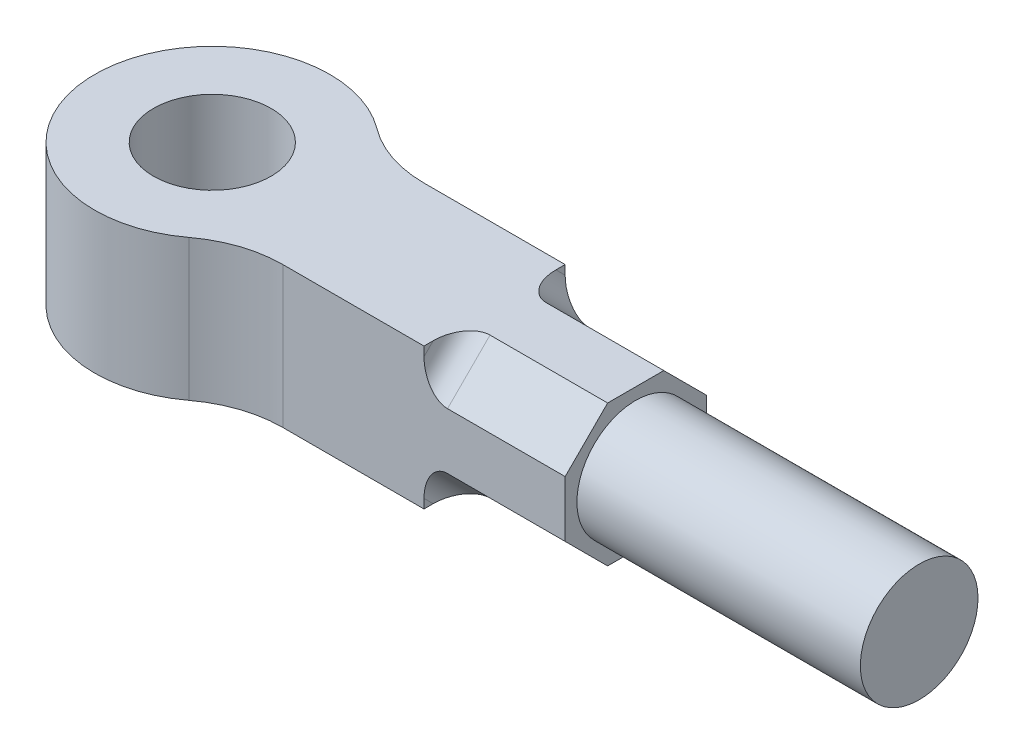
ISO-10303-21;
HEADER;
FILE_DESCRIPTION(('STEP AP214'),'2;1');
FILE_NAME('part.step','',(''),(''),'','','');
FILE_SCHEMA(('AUTOMOTIVE_DESIGN { 1 0 10303 214 1 1 1 1 }'));
ENDSEC;
DATA;
#1=APPLICATION_CONTEXT('core data for automotive mechanical design processes');
#2=APPLICATION_PROTOCOL_DEFINITION('international standard','automotive_design',2000,#1);
#3=PRODUCT_CONTEXT('',#1,'mechanical');
#4=PRODUCT('Part','Part','',(#3));
#5=PRODUCT_RELATED_PRODUCT_CATEGORY('part','',(#4));
#6=PRODUCT_DEFINITION_FORMATION('','',#4);
#7=PRODUCT_DEFINITION_CONTEXT('part definition',#1,'design');
#8=PRODUCT_DEFINITION('design','',#6,#7);
#9=PRODUCT_DEFINITION_SHAPE('','',#8);
#10=(LENGTH_UNIT() NAMED_UNIT(*) SI_UNIT(.MILLI.,.METRE.));
#11=(NAMED_UNIT(*) PLANE_ANGLE_UNIT() SI_UNIT($,.RADIAN.));
#12=(NAMED_UNIT(*) SI_UNIT($,.STERADIAN.) SOLID_ANGLE_UNIT());
#13=UNCERTAINTY_MEASURE_WITH_UNIT(LENGTH_MEASURE(1.E-05),#10,'distance_accuracy_value','');
#14=(GEOMETRIC_REPRESENTATION_CONTEXT(3) GLOBAL_UNCERTAINTY_ASSIGNED_CONTEXT((#13)) GLOBAL_UNIT_ASSIGNED_CONTEXT((#10,
#11,#12)) REPRESENTATION_CONTEXT('',''));
#15=CARTESIAN_POINT('',(0.,0.,0.));
#16=DIRECTION('',(0.,0.,1.));
#17=DIRECTION('',(1.,0.,0.));
#18=AXIS2_PLACEMENT_3D('',#15,#16,#17);
#19=CARTESIAN_POINT('',(60.,60.,-80.));
#20=DIRECTION('',(0.,1.,0.));
#21=DIRECTION('',(0.,0.,1.));
#22=AXIS2_PLACEMENT_3D('',#19,#20,#21);
#23=PLANE('',#22);
#24=CARTESIAN_POINT('',(0.,60.,0.));
#25=DIRECTION('',(0.,1.,0.));
#26=DIRECTION('',(0.,0.,1.));
#27=AXIS2_PLACEMENT_3D('',#24,#25,#26);
#28=CIRCLE('',#27,25.);
#29=CARTESIAN_POINT('',(0.,60.,25.));
#30=VERTEX_POINT('',#29);
#31=EDGE_CURVE('E289',#30,#30,#28,.T.);
#32=ORIENTED_EDGE('',*,*,#31,.F.);
#33=EDGE_LOOP('',(#32));
#34=FACE_BOUND('',#33,.T.);
#35=DIRECTION('',(0.,0.,-1.));
#36=VECTOR('',#35,1.);
#37=CARTESIAN_POINT('',(180.,60.,-30.));
#38=LINE('',#37,#36);
#39=CARTESIAN_POINT('',(180.,60.,11.9399999999999));
#40=VERTEX_POINT('',#39);
#41=CARTESIAN_POINT('',(180.,60.,-11.94));
#42=VERTEX_POINT('',#41);
#43=EDGE_CURVE('E303',#40,#42,#38,.T.);
#44=ORIENTED_EDGE('',*,*,#43,.T.);
#45=DIRECTION('',(1.,0.,0.));
#46=VECTOR('',#45,1.);
#47=CARTESIAN_POINT('',(120.,60.,-11.94));
#48=LINE('',#47,#46);
#49=CARTESIAN_POINT('',(130.,60.,-11.94));
#50=VERTEX_POINT('',#49);
#51=EDGE_CURVE('E290',#50,#42,#48,.T.);
#52=ORIENTED_EDGE('',*,*,#51,.F.);
#53=CARTESIAN_POINT('',(130.,60.,-26.0821356237309));
#54=DIRECTION('',(0.,1.,0.));
#55=DIRECTION('',(0.,0.,-1.));
#56=AXIS2_PLACEMENT_3D('',#53,#54,#55);
#57=ELLIPSE('',#56,14.1421356237309,10.);
#58=CARTESIAN_POINT('',(120.,60.,-26.0821356237309));
#59=VERTEX_POINT('',#58);
#60=EDGE_CURVE('E47',#50,#59,#57,.F.);
#61=ORIENTED_EDGE('',*,*,#60,.T.);
#62=DIRECTION('',(0.,0.,1.));
#63=VECTOR('',#62,1.);
#64=CARTESIAN_POINT('',(120.,60.,0.));
#65=LINE('',#64,#63);
#66=CARTESIAN_POINT('',(120.,60.,-30.));
#67=VERTEX_POINT('',#66);
#68=EDGE_CURVE('E333',#67,#59,#65,.T.);
#69=ORIENTED_EDGE('',*,*,#68,.F.);
#70=DIRECTION('',(-1.,0.,0.));
#71=VECTOR('',#70,1.);
#72=CARTESIAN_POINT('',(60.,60.,-30.));
#73=LINE('',#72,#71);
#74=CARTESIAN_POINT('',(60.,60.,-30.));
#75=VERTEX_POINT('',#74);
#76=EDGE_CURVE('E209',#67,#75,#73,.T.);
#77=ORIENTED_EDGE('',*,*,#76,.T.);
#78=CARTESIAN_POINT('',(60.,60.,-80.));
#79=DIRECTION('',(0.,-1.,0.));
#80=DIRECTION('',(0.,0.,1.));
#81=AXIS2_PLACEMENT_3D('',#78,#79,#80);
#82=CIRCLE('',#81,50.);
#83=CARTESIAN_POINT('',(30.,60.,-40.));
#84=VERTEX_POINT('',#83);
#85=EDGE_CURVE('E200',#75,#84,#82,.T.);
#86=ORIENTED_EDGE('',*,*,#85,.T.);
#87=CARTESIAN_POINT('',(0.,60.,0.));
#88=DIRECTION('',(0.,1.,0.));
#89=DIRECTION('',(0.,0.,1.));
#90=AXIS2_PLACEMENT_3D('',#87,#88,#89);
#91=CIRCLE('',#90,50.);
#92=CARTESIAN_POINT('',(30.,60.,40.));
#93=VERTEX_POINT('',#92);
#94=EDGE_CURVE('E296',#84,#93,#91,.T.);
#95=ORIENTED_EDGE('',*,*,#94,.T.);
#96=CARTESIAN_POINT('',(60.,60.,80.));
#97=DIRECTION('',(0.,-1.,0.));
#98=DIRECTION('',(0.,0.,-1.));
#99=AXIS2_PLACEMENT_3D('',#96,#97,#98);
#100=CIRCLE('',#99,50.);
#101=CARTESIAN_POINT('',(60.,60.,30.));
#102=VERTEX_POINT('',#101);
#103=EDGE_CURVE('E297',#93,#102,#100,.T.);
#104=ORIENTED_EDGE('',*,*,#103,.T.);
#105=DIRECTION('',(1.,0.,0.));
#106=VECTOR('',#105,1.);
#107=CARTESIAN_POINT('',(60.,60.,30.));
#108=LINE('',#107,#106);
#109=CARTESIAN_POINT('',(120.,60.,30.));
#110=VERTEX_POINT('',#109);
#111=EDGE_CURVE('E305',#102,#110,#108,.T.);
#112=ORIENTED_EDGE('',*,*,#111,.T.);
#113=DIRECTION('',(0.,0.,1.));
#114=VECTOR('',#113,1.);
#115=CARTESIAN_POINT('',(120.,60.,0.));
#116=LINE('',#115,#114);
#117=CARTESIAN_POINT('',(120.,60.,26.0821356237309));
#118=VERTEX_POINT('',#117);
#119=EDGE_CURVE('E259',#118,#110,#116,.T.);
#120=ORIENTED_EDGE('',*,*,#119,.F.);
#121=CARTESIAN_POINT('',(130.,60.,26.0821356237309));
#122=DIRECTION('',(0.,1.,0.));
#123=DIRECTION('',(0.,0.,-1.));
#124=AXIS2_PLACEMENT_3D('',#121,#122,#123);
#125=ELLIPSE('',#124,14.142135623731,10.);
#126=CARTESIAN_POINT('',(130.,60.,11.94));
#127=VERTEX_POINT('',#126);
#128=EDGE_CURVE('E253',#118,#127,#125,.F.);
#129=ORIENTED_EDGE('',*,*,#128,.T.);
#130=DIRECTION('',(1.,0.,0.));
#131=VECTOR('',#130,1.);
#132=CARTESIAN_POINT('',(120.,60.,11.94));
#133=LINE('',#132,#131);
#134=EDGE_CURVE('E258',#127,#40,#133,.T.);
#135=ORIENTED_EDGE('',*,*,#134,.T.);
#136=EDGE_LOOP('',(#44,#52,#61,#69,#77,#86,#95,#104,#112,#120,#129,#135));
#137=FACE_BOUND('',#136,.T.);
#138=ADVANCED_FACE('F41',(#34,#137),#23,.T.);
#139=CARTESIAN_POINT('',(60.,0.,-80.));
#140=DIRECTION('',(0.,1.,0.));
#141=DIRECTION('',(0.,0.,1.));
#142=AXIS2_PLACEMENT_3D('',#139,#140,#141);
#143=PLANE('',#142);
#144=CARTESIAN_POINT('',(0.,0.,0.));
#145=DIRECTION('',(0.,1.,0.));
#146=DIRECTION('',(0.,0.,1.));
#147=AXIS2_PLACEMENT_3D('',#144,#145,#146);
#148=CIRCLE('',#147,25.);
#149=CARTESIAN_POINT('',(0.,0.,25.));
#150=VERTEX_POINT('',#149);
#151=EDGE_CURVE('E287',#150,#150,#148,.T.);
#152=ORIENTED_EDGE('',*,*,#151,.T.);
#153=EDGE_LOOP('',(#152));
#154=FACE_BOUND('',#153,.T.);
#155=DIRECTION('',(1.,0.,0.));
#156=VECTOR('',#155,1.);
#157=CARTESIAN_POINT('',(120.,0.,11.94));
#158=LINE('',#157,#156);
#159=CARTESIAN_POINT('',(130.,0.,11.94));
#160=VERTEX_POINT('',#159);
#161=CARTESIAN_POINT('',(180.,0.,11.94));
#162=VERTEX_POINT('',#161);
#163=EDGE_CURVE('E324',#160,#162,#158,.T.);
#164=ORIENTED_EDGE('',*,*,#163,.F.);
#165=CARTESIAN_POINT('',(130.,0.,26.082135623731));
#166=DIRECTION('',(0.,1.,0.));
#167=DIRECTION('',(0.,0.,1.));
#168=AXIS2_PLACEMENT_3D('',#165,#166,#167);
#169=ELLIPSE('',#168,14.1421356237309,10.);
#170=CARTESIAN_POINT('',(120.,0.,26.082135623731));
#171=VERTEX_POINT('',#170);
#172=EDGE_CURVE('E242',#160,#171,#169,.T.);
#173=ORIENTED_EDGE('',*,*,#172,.T.);
#174=DIRECTION('',(0.,0.,-1.));
#175=VECTOR('',#174,1.);
#176=CARTESIAN_POINT('',(120.,0.,0.));
#177=LINE('',#176,#175);
#178=CARTESIAN_POINT('',(120.,0.,30.));
#179=VERTEX_POINT('',#178);
#180=EDGE_CURVE('E317',#179,#171,#177,.T.);
#181=ORIENTED_EDGE('',*,*,#180,.F.);
#182=DIRECTION('',(1.,0.,0.));
#183=VECTOR('',#182,1.);
#184=CARTESIAN_POINT('',(60.,0.,30.));
#185=LINE('',#184,#183);
#186=CARTESIAN_POINT('',(60.,0.,30.));
#187=VERTEX_POINT('',#186);
#188=EDGE_CURVE('E197',#187,#179,#185,.T.);
#189=ORIENTED_EDGE('',*,*,#188,.F.);
#190=CARTESIAN_POINT('',(60.,0.,80.));
#191=DIRECTION('',(0.,-1.,0.));
#192=DIRECTION('',(0.,0.,-1.));
#193=AXIS2_PLACEMENT_3D('',#190,#191,#192);
#194=CIRCLE('',#193,50.);
#195=CARTESIAN_POINT('',(30.,0.,40.));
#196=VERTEX_POINT('',#195);
#197=EDGE_CURVE('E205',#196,#187,#194,.T.);
#198=ORIENTED_EDGE('',*,*,#197,.F.);
#199=CARTESIAN_POINT('',(0.,0.,0.));
#200=DIRECTION('',(0.,1.,0.));
#201=DIRECTION('',(0.,0.,1.));
#202=AXIS2_PLACEMENT_3D('',#199,#200,#201);
#203=CIRCLE('',#202,50.);
#204=CARTESIAN_POINT('',(30.,0.,-40.));
#205=VERTEX_POINT('',#204);
#206=EDGE_CURVE('E310',#205,#196,#203,.T.);
#207=ORIENTED_EDGE('',*,*,#206,.F.);
#208=CARTESIAN_POINT('',(60.,0.,-80.));
#209=DIRECTION('',(0.,-1.,0.));
#210=DIRECTION('',(0.,0.,1.));
#211=AXIS2_PLACEMENT_3D('',#208,#209,#210);
#212=CIRCLE('',#211,50.);
#213=CARTESIAN_POINT('',(60.,0.,-30.));
#214=VERTEX_POINT('',#213);
#215=EDGE_CURVE('E291',#214,#205,#212,.T.);
#216=ORIENTED_EDGE('',*,*,#215,.F.);
#217=DIRECTION('',(-1.,0.,0.));
#218=VECTOR('',#217,1.);
#219=CARTESIAN_POINT('',(60.,0.,-30.));
#220=LINE('',#219,#218);
#221=CARTESIAN_POINT('',(120.,0.,-30.));
#222=VERTEX_POINT('',#221);
#223=EDGE_CURVE('E198',#222,#214,#220,.T.);
#224=ORIENTED_EDGE('',*,*,#223,.F.);
#225=DIRECTION('',(0.,0.,-1.));
#226=VECTOR('',#225,1.);
#227=CARTESIAN_POINT('',(120.,0.,0.));
#228=LINE('',#227,#226);
#229=CARTESIAN_POINT('',(120.,0.,-26.0821356237309));
#230=VERTEX_POINT('',#229);
#231=EDGE_CURVE('E190',#230,#222,#228,.T.);
#232=ORIENTED_EDGE('',*,*,#231,.F.);
#233=CARTESIAN_POINT('',(130.,0.,-26.0821356237309));
#234=DIRECTION('',(0.,1.,0.));
#235=DIRECTION('',(0.,0.,1.));
#236=AXIS2_PLACEMENT_3D('',#233,#234,#235);
#237=ELLIPSE('',#236,14.142135623731,10.);
#238=CARTESIAN_POINT('',(130.,0.,-11.9399999999999));
#239=VERTEX_POINT('',#238);
#240=EDGE_CURVE('E171',#230,#239,#237,.T.);
#241=ORIENTED_EDGE('',*,*,#240,.T.);
#242=DIRECTION('',(1.,0.,0.));
#243=VECTOR('',#242,1.);
#244=CARTESIAN_POINT('',(120.,0.,-11.9399999999999));
#245=LINE('',#244,#243);
#246=CARTESIAN_POINT('',(180.,0.,-11.9399999999999));
#247=VERTEX_POINT('',#246);
#248=EDGE_CURVE('E164',#239,#247,#245,.T.);
#249=ORIENTED_EDGE('',*,*,#248,.T.);
#250=DIRECTION('',(0.,0.,-1.));
#251=VECTOR('',#250,1.);
#252=CARTESIAN_POINT('',(180.,0.,-30.));
#253=LINE('',#252,#251);
#254=EDGE_CURVE('E168',#162,#247,#253,.T.);
#255=ORIENTED_EDGE('',*,*,#254,.F.);
#256=EDGE_LOOP('',(#164,#173,#181,#189,#198,#207,#216,#224,#232,#241,#249,#255));
#257=FACE_BOUND('',#256,.T.);
#258=ADVANCED_FACE('F169',(#154,#257),#143,.F.);
#259=CARTESIAN_POINT('',(60.,60.,30.));
#260=DIRECTION('',(0.,0.,-1.));
#261=DIRECTION('',(-1.,0.,0.));
#262=AXIS2_PLACEMENT_3D('',#259,#260,#261);
#263=PLANE('',#262);
#264=DIRECTION('',(0.,-1.,0.));
#265=VECTOR('',#264,1.);
#266=CARTESIAN_POINT('',(120.,0.,30.));
#267=LINE('',#266,#265);
#268=CARTESIAN_POINT('',(120.,3.91786437626909,30.));
#269=VERTEX_POINT('',#268);
#270=EDGE_CURVE('E323',#269,#179,#267,.T.);
#271=ORIENTED_EDGE('',*,*,#270,.F.);
#272=CARTESIAN_POINT('',(130.,3.91786437626906,30.));
#273=DIRECTION('',(0.,0.,-1.));
#274=DIRECTION('',(0.,1.,0.));
#275=AXIS2_PLACEMENT_3D('',#272,#273,#274);
#276=ELLIPSE('',#275,14.142135623731,10.);
#277=CARTESIAN_POINT('',(130.,18.0600000000001,30.));
#278=VERTEX_POINT('',#277);
#279=EDGE_CURVE('E250',#269,#278,#276,.T.);
#280=ORIENTED_EDGE('',*,*,#279,.T.);
#281=DIRECTION('',(1.,0.,0.));
#282=VECTOR('',#281,1.);
#283=CARTESIAN_POINT('',(120.,18.0600000000001,30.));
#284=LINE('',#283,#282);
#285=CARTESIAN_POINT('',(180.,18.0600000000001,30.));
#286=VERTEX_POINT('',#285);
#287=EDGE_CURVE('E325',#278,#286,#284,.T.);
#288=ORIENTED_EDGE('',*,*,#287,.T.);
#289=DIRECTION('',(0.,-1.,0.));
#290=VECTOR('',#289,1.);
#291=CARTESIAN_POINT('',(180.,60.,30.));
#292=LINE('',#291,#290);
#293=CARTESIAN_POINT('',(180.,41.94,30.));
#294=VERTEX_POINT('',#293);
#295=EDGE_CURVE('E215',#294,#286,#292,.T.);
#296=ORIENTED_EDGE('',*,*,#295,.F.);
#297=DIRECTION('',(1.,0.,0.));
#298=VECTOR('',#297,1.);
#299=CARTESIAN_POINT('',(120.,41.94,30.));
#300=LINE('',#299,#298);
#301=CARTESIAN_POINT('',(130.,41.94,30.));
#302=VERTEX_POINT('',#301);
#303=EDGE_CURVE('E267',#302,#294,#300,.T.);
#304=ORIENTED_EDGE('',*,*,#303,.F.);
#305=CARTESIAN_POINT('',(130.,56.0821356237309,30.));
#306=DIRECTION('',(0.,0.,-1.));
#307=DIRECTION('',(0.,1.,0.));
#308=AXIS2_PLACEMENT_3D('',#305,#306,#307);
#309=ELLIPSE('',#308,14.1421356237309,10.);
#310=CARTESIAN_POINT('',(120.,56.0821356237309,30.));
#311=VERTEX_POINT('',#310);
#312=EDGE_CURVE('E248',#302,#311,#309,.T.);
#313=ORIENTED_EDGE('',*,*,#312,.T.);
#314=DIRECTION('',(0.,-1.,0.));
#315=VECTOR('',#314,1.);
#316=CARTESIAN_POINT('',(120.,0.,30.));
#317=LINE('',#316,#315);
#318=EDGE_CURVE('E269',#110,#311,#317,.T.);
#319=ORIENTED_EDGE('',*,*,#318,.F.);
#320=ORIENTED_EDGE('',*,*,#111,.F.);
#321=DIRECTION('',(0.,-1.,0.));
#322=VECTOR('',#321,1.);
#323=CARTESIAN_POINT('',(60.,60.,30.));
#324=LINE('',#323,#322);
#325=EDGE_CURVE('E212',#102,#187,#324,.T.);
#326=ORIENTED_EDGE('',*,*,#325,.T.);
#327=ORIENTED_EDGE('',*,*,#188,.T.);
#328=EDGE_LOOP('',(#271,#280,#288,#296,#304,#313,#319,#320,#326,#327));
#329=FACE_BOUND('',#328,.T.);
#330=ADVANCED_FACE('F280',(#329),#263,.F.);
#331=CARTESIAN_POINT('',(180.,60.,-30.));
#332=DIRECTION('',(-1.,0.,0.));
#333=DIRECTION('',(0.,0.,1.));
#334=AXIS2_PLACEMENT_3D('',#331,#332,#333);
#335=PLANE('',#334);
#336=CARTESIAN_POINT('',(180.,30.,0.));
#337=DIRECTION('',(1.,0.,0.));
#338=DIRECTION('',(0.,0.,-1.));
#339=AXIS2_PLACEMENT_3D('',#336,#337,#338);
#340=CIRCLE('',#339,25.);
#341=CARTESIAN_POINT('',(180.,30.,-25.));
#342=VERTEX_POINT('',#341);
#343=EDGE_CURVE('E224',#342,#342,#340,.T.);
#344=ORIENTED_EDGE('',*,*,#343,.F.);
#345=EDGE_LOOP('',(#344));
#346=FACE_BOUND('',#345,.T.);
#347=DIRECTION('',(0.,0.707106781186549,0.707106781186546));
#348=VECTOR('',#347,1.);
#349=CARTESIAN_POINT('',(180.,35.9699999999999,-35.97));
#350=LINE('',#349,#348);
#351=CARTESIAN_POINT('',(180.,41.9399999999999,-30.));
#352=VERTEX_POINT('',#351);
#353=EDGE_CURVE('E329',#352,#42,#350,.T.);
#354=ORIENTED_EDGE('',*,*,#353,.T.);
#355=ORIENTED_EDGE('',*,*,#43,.F.);
#356=DIRECTION('',(0.,-0.707106781186546,0.707106781186549));
#357=VECTOR('',#356,1.);
#358=CARTESIAN_POINT('',(180.,35.9700000000001,35.9699999999999));
#359=LINE('',#358,#357);
#360=EDGE_CURVE('E270',#40,#294,#359,.T.);
#361=ORIENTED_EDGE('',*,*,#360,.T.);
#362=ORIENTED_EDGE('',*,*,#295,.T.);
#363=DIRECTION('',(0.,-0.707106781186549,-0.707106781186546));
#364=VECTOR('',#363,1.);
#365=CARTESIAN_POINT('',(180.,-5.97000000000004,5.96999999999998));
#366=LINE('',#365,#364);
#367=EDGE_CURVE('E194',#286,#162,#366,.T.);
#368=ORIENTED_EDGE('',*,*,#367,.T.);
#369=ORIENTED_EDGE('',*,*,#254,.T.);
#370=DIRECTION('',(0.,0.707106781186546,-0.707106781186549));
#371=VECTOR('',#370,1.);
#372=CARTESIAN_POINT('',(180.,-5.96999999999993,-5.96999999999998));
#373=LINE('',#372,#371);
#374=CARTESIAN_POINT('',(180.,18.06,-30.));
#375=VERTEX_POINT('',#374);
#376=EDGE_CURVE('E182',#247,#375,#373,.T.);
#377=ORIENTED_EDGE('',*,*,#376,.T.);
#378=DIRECTION('',(0.,-1.,0.));
#379=VECTOR('',#378,1.);
#380=CARTESIAN_POINT('',(180.,60.,-30.));
#381=LINE('',#380,#379);
#382=EDGE_CURVE('E207',#352,#375,#381,.T.);
#383=ORIENTED_EDGE('',*,*,#382,.F.);
#384=EDGE_LOOP('',(#354,#355,#361,#362,#368,#369,#377,#383));
#385=FACE_BOUND('',#384,.T.);
#386=ADVANCED_FACE('F195',(#346,#385),#335,.F.);
#387=CARTESIAN_POINT('',(60.,60.,-30.));
#388=DIRECTION('',(0.,0.,1.));
#389=DIRECTION('',(1.,0.,0.));
#390=AXIS2_PLACEMENT_3D('',#387,#388,#389);
#391=PLANE('',#390);
#392=DIRECTION('',(0.,1.,0.));
#393=VECTOR('',#392,1.);
#394=CARTESIAN_POINT('',(120.,0.,-30.));
#395=LINE('',#394,#393);
#396=CARTESIAN_POINT('',(120.,56.0821356237309,-30.));
#397=VERTEX_POINT('',#396);
#398=EDGE_CURVE('E335',#397,#67,#395,.T.);
#399=ORIENTED_EDGE('',*,*,#398,.F.);
#400=CARTESIAN_POINT('',(130.,56.0821356237309,-30.));
#401=DIRECTION('',(0.,0.,1.));
#402=DIRECTION('',(0.,-1.,0.));
#403=AXIS2_PLACEMENT_3D('',#400,#401,#402);
#404=ELLIPSE('',#403,14.142135623731,10.);
#405=CARTESIAN_POINT('',(130.,41.9399999999999,-30.));
#406=VERTEX_POINT('',#405);
#407=EDGE_CURVE('E11',#397,#406,#404,.T.);
#408=ORIENTED_EDGE('',*,*,#407,.T.);
#409=DIRECTION('',(1.,0.,0.));
#410=VECTOR('',#409,1.);
#411=CARTESIAN_POINT('',(120.,41.9399999999999,-30.));
#412=LINE('',#411,#410);
#413=EDGE_CURVE('E339',#406,#352,#412,.T.);
#414=ORIENTED_EDGE('',*,*,#413,.T.);
#415=ORIENTED_EDGE('',*,*,#382,.T.);
#416=DIRECTION('',(1.,0.,0.));
#417=VECTOR('',#416,1.);
#418=CARTESIAN_POINT('',(120.,18.06,-30.));
#419=LINE('',#418,#417);
#420=CARTESIAN_POINT('',(130.,18.06,-30.));
#421=VERTEX_POINT('',#420);
#422=EDGE_CURVE('E180',#421,#375,#419,.T.);
#423=ORIENTED_EDGE('',*,*,#422,.F.);
#424=CARTESIAN_POINT('',(130.,3.9178643762691,-30.));
#425=DIRECTION('',(0.,0.,1.));
#426=DIRECTION('',(0.,-1.,0.));
#427=AXIS2_PLACEMENT_3D('',#424,#425,#426);
#428=ELLIPSE('',#427,14.1421356237309,10.);
#429=CARTESIAN_POINT('',(120.,3.91786437626907,-30.));
#430=VERTEX_POINT('',#429);
#431=EDGE_CURVE('E245',#421,#430,#428,.T.);
#432=ORIENTED_EDGE('',*,*,#431,.T.);
#433=DIRECTION('',(0.,1.,0.));
#434=VECTOR('',#433,1.);
#435=CARTESIAN_POINT('',(120.,0.,-30.));
#436=LINE('',#435,#434);
#437=EDGE_CURVE('E177',#222,#430,#436,.T.);
#438=ORIENTED_EDGE('',*,*,#437,.F.);
#439=ORIENTED_EDGE('',*,*,#223,.T.);
#440=DIRECTION('',(0.,-1.,0.));
#441=VECTOR('',#440,1.);
#442=CARTESIAN_POINT('',(60.,60.,-30.));
#443=LINE('',#442,#441);
#444=EDGE_CURVE('E206',#75,#214,#443,.T.);
#445=ORIENTED_EDGE('',*,*,#444,.F.);
#446=ORIENTED_EDGE('',*,*,#76,.F.);
#447=EDGE_LOOP('',(#399,#408,#414,#415,#423,#432,#438,#439,#445,#446));
#448=FACE_BOUND('',#447,.T.);
#449=ADVANCED_FACE('F350',(#448),#391,.F.);
#450=CARTESIAN_POINT('',(60.,60.,-80.));
#451=DIRECTION('',(0.,-1.,0.));
#452=DIRECTION('',(0.,0.,-1.));
#453=AXIS2_PLACEMENT_3D('',#450,#451,#452);
#454=CYLINDRICAL_SURFACE('',#453,50.);
#455=ORIENTED_EDGE('',*,*,#215,.T.);
#456=DIRECTION('',(0.,-1.,0.));
#457=VECTOR('',#456,1.);
#458=CARTESIAN_POINT('',(30.,60.,-40.));
#459=LINE('',#458,#457);
#460=EDGE_CURVE('E219',#84,#205,#459,.T.);
#461=ORIENTED_EDGE('',*,*,#460,.F.);
#462=ORIENTED_EDGE('',*,*,#85,.F.);
#463=ORIENTED_EDGE('',*,*,#444,.T.);
#464=EDGE_LOOP('',(#455,#461,#462,#463));
#465=FACE_BOUND('',#464,.T.);
#466=ADVANCED_FACE('F376',(#465),#454,.F.);
#467=CARTESIAN_POINT('',(0.,60.,0.));
#468=DIRECTION('',(0.,-1.,0.));
#469=DIRECTION('',(0.,0.,-1.));
#470=AXIS2_PLACEMENT_3D('',#467,#468,#469);
#471=CYLINDRICAL_SURFACE('',#470,50.);
#472=ORIENTED_EDGE('',*,*,#206,.T.);
#473=DIRECTION('',(0.,-1.,0.));
#474=VECTOR('',#473,1.);
#475=CARTESIAN_POINT('',(30.,60.,40.));
#476=LINE('',#475,#474);
#477=EDGE_CURVE('E220',#93,#196,#476,.T.);
#478=ORIENTED_EDGE('',*,*,#477,.F.);
#479=ORIENTED_EDGE('',*,*,#94,.F.);
#480=ORIENTED_EDGE('',*,*,#460,.T.);
#481=EDGE_LOOP('',(#472,#478,#479,#480));
#482=FACE_BOUND('',#481,.T.);
#483=ADVANCED_FACE('F550',(#482),#471,.T.);
#484=CARTESIAN_POINT('',(60.,60.,80.));
#485=DIRECTION('',(0.,-1.,0.));
#486=DIRECTION('',(0.,0.,-1.));
#487=AXIS2_PLACEMENT_3D('',#484,#485,#486);
#488=CYLINDRICAL_SURFACE('',#487,50.);
#489=ORIENTED_EDGE('',*,*,#197,.T.);
#490=ORIENTED_EDGE('',*,*,#325,.F.);
#491=ORIENTED_EDGE('',*,*,#103,.F.);
#492=ORIENTED_EDGE('',*,*,#477,.T.);
#493=EDGE_LOOP('',(#489,#490,#491,#492));
#494=FACE_BOUND('',#493,.T.);
#495=ADVANCED_FACE('F311',(#494),#488,.F.);
#496=CARTESIAN_POINT('',(0.,60.,0.));
#497=DIRECTION('',(0.,-1.,0.));
#498=DIRECTION('',(0.,0.,-1.));
#499=AXIS2_PLACEMENT_3D('',#496,#497,#498);
#500=CYLINDRICAL_SURFACE('',#499,25.);
#501=ORIENTED_EDGE('',*,*,#31,.T.);
#502=EDGE_LOOP('',(#501));
#503=FACE_BOUND('',#502,.T.);
#504=ORIENTED_EDGE('',*,*,#151,.F.);
#505=EDGE_LOOP('',(#504));
#506=FACE_BOUND('',#505,.T.);
#507=ADVANCED_FACE('F393',(#503,#506),#500,.F.);
#508=CARTESIAN_POINT('',(120.,-5.96999999999993,-5.96999999999996));
#509=DIRECTION('',(0.,-0.707106781186549,-0.707106781186546));
#510=DIRECTION('',(0.,0.707106781186546,-0.707106781186549));
#511=AXIS2_PLACEMENT_3D('',#508,#509,#510);
#512=PLANE('',#511);
#513=ORIENTED_EDGE('',*,*,#248,.F.);
#514=DIRECTION('',(0.,0.707106781186546,-0.707106781186549));
#515=VECTOR('',#514,1.);
#516=CARTESIAN_POINT('',(130.,18.06,-30.));
#517=LINE('',#516,#515);
#518=EDGE_CURVE('E221',#239,#421,#517,.T.);
#519=ORIENTED_EDGE('',*,*,#518,.T.);
#520=ORIENTED_EDGE('',*,*,#422,.T.);
#521=ORIENTED_EDGE('',*,*,#376,.F.);
#522=EDGE_LOOP('',(#513,#519,#520,#521));
#523=FACE_BOUND('',#522,.T.);
#524=ADVANCED_FACE('F185',(#523),#512,.T.);
#525=CARTESIAN_POINT('',(120.,0.,0.));
#526=DIRECTION('',(1.,0.,0.));
#527=DIRECTION('',(0.,0.,-1.));
#528=AXIS2_PLACEMENT_3D('',#525,#526,#527);
#529=PLANE('',#528);
#530=ORIENTED_EDGE('',*,*,#437,.T.);
#531=DIRECTION('',(0.,0.707106781186546,-0.707106781186549));
#532=VECTOR('',#531,1.);
#533=CARTESIAN_POINT('',(120.,-7.07106781186549,-19.0110678118654));
#534=LINE('',#533,#532);
#535=EDGE_CURVE('E228',#430,#230,#534,.F.);
#536=ORIENTED_EDGE('',*,*,#535,.T.);
#537=ORIENTED_EDGE('',*,*,#231,.T.);
#538=EDGE_LOOP('',(#530,#536,#537));
#539=FACE_BOUND('',#538,.T.);
#540=ADVANCED_FACE('F403',(#539),#529,.T.);
#541=CARTESIAN_POINT('',(120.,35.9699999999999,-35.97));
#542=DIRECTION('',(0.,0.707106781186546,-0.707106781186549));
#543=DIRECTION('',(0.,0.707106781186549,0.707106781186546));
#544=AXIS2_PLACEMENT_3D('',#541,#542,#543);
#545=PLANE('',#544);
#546=ORIENTED_EDGE('',*,*,#413,.F.);
#547=DIRECTION('',(0.,0.707106781186549,0.707106781186546));
#548=VECTOR('',#547,1.);
#549=CARTESIAN_POINT('',(130.,60.,-11.94));
#550=LINE('',#549,#548);
#551=EDGE_CURVE('E236',#406,#50,#550,.T.);
#552=ORIENTED_EDGE('',*,*,#551,.T.);
#553=ORIENTED_EDGE('',*,*,#51,.T.);
#554=ORIENTED_EDGE('',*,*,#353,.F.);
#555=EDGE_LOOP('',(#546,#552,#553,#554));
#556=FACE_BOUND('',#555,.T.);
#557=ADVANCED_FACE('F349',(#556),#545,.T.);
#558=CARTESIAN_POINT('',(120.,0.,0.));
#559=DIRECTION('',(1.,0.,0.));
#560=DIRECTION('',(0.,0.,-1.));
#561=AXIS2_PLACEMENT_3D('',#558,#559,#560);
#562=PLANE('',#561);
#563=ORIENTED_EDGE('',*,*,#68,.T.);
#564=DIRECTION('',(0.,0.707106781186549,0.707106781186546));
#565=VECTOR('',#564,1.);
#566=CARTESIAN_POINT('',(120.,49.0110678118654,-37.0710678118655));
#567=LINE('',#566,#565);
#568=EDGE_CURVE('E65',#59,#397,#567,.F.);
#569=ORIENTED_EDGE('',*,*,#568,.T.);
#570=ORIENTED_EDGE('',*,*,#398,.T.);
#571=EDGE_LOOP('',(#563,#569,#570));
#572=FACE_BOUND('',#571,.T.);
#573=ADVANCED_FACE('F345',(#572),#562,.T.);
#574=CARTESIAN_POINT('',(120.,35.9700000000001,35.9699999999999));
#575=DIRECTION('',(0.,0.707106781186549,0.707106781186546));
#576=DIRECTION('',(0.,-0.707106781186546,0.707106781186549));
#577=AXIS2_PLACEMENT_3D('',#574,#575,#576);
#578=PLANE('',#577);
#579=ORIENTED_EDGE('',*,*,#134,.F.);
#580=DIRECTION('',(0.,-0.707106781186546,0.707106781186549));
#581=VECTOR('',#580,1.);
#582=CARTESIAN_POINT('',(130.,41.94,30.));
#583=LINE('',#582,#581);
#584=EDGE_CURVE('E232',#127,#302,#583,.T.);
#585=ORIENTED_EDGE('',*,*,#584,.T.);
#586=ORIENTED_EDGE('',*,*,#303,.T.);
#587=ORIENTED_EDGE('',*,*,#360,.F.);
#588=EDGE_LOOP('',(#579,#585,#586,#587));
#589=FACE_BOUND('',#588,.T.);
#590=ADVANCED_FACE('F262',(#589),#578,.T.);
#591=CARTESIAN_POINT('',(120.,0.,0.));
#592=DIRECTION('',(1.,0.,0.));
#593=DIRECTION('',(0.,0.,-1.));
#594=AXIS2_PLACEMENT_3D('',#591,#592,#593);
#595=PLANE('',#594);
#596=ORIENTED_EDGE('',*,*,#318,.T.);
#597=DIRECTION('',(0.,-0.707106781186546,0.707106781186549));
#598=VECTOR('',#597,1.);
#599=CARTESIAN_POINT('',(120.,67.0710678118655,19.0110678118654));
#600=LINE('',#599,#598);
#601=EDGE_CURVE('E237',#311,#118,#600,.F.);
#602=ORIENTED_EDGE('',*,*,#601,.T.);
#603=ORIENTED_EDGE('',*,*,#119,.T.);
#604=EDGE_LOOP('',(#596,#602,#603));
#605=FACE_BOUND('',#604,.T.);
#606=ADVANCED_FACE('F283',(#605),#595,.T.);
#607=CARTESIAN_POINT('',(120.,-5.97000000000004,5.97000000000001));
#608=DIRECTION('',(0.,-0.707106781186546,0.707106781186549));
#609=DIRECTION('',(0.,-0.707106781186549,-0.707106781186546));
#610=AXIS2_PLACEMENT_3D('',#607,#608,#609);
#611=PLANE('',#610);
#612=ORIENTED_EDGE('',*,*,#287,.F.);
#613=DIRECTION('',(0.,-0.707106781186549,-0.707106781186546));
#614=VECTOR('',#613,1.);
#615=CARTESIAN_POINT('',(130.,0.,11.94));
#616=LINE('',#615,#614);
#617=EDGE_CURVE('E226',#278,#160,#616,.T.);
#618=ORIENTED_EDGE('',*,*,#617,.T.);
#619=ORIENTED_EDGE('',*,*,#163,.T.);
#620=ORIENTED_EDGE('',*,*,#367,.F.);
#621=EDGE_LOOP('',(#612,#618,#619,#620));
#622=FACE_BOUND('',#621,.T.);
#623=ADVANCED_FACE('F397',(#622),#611,.T.);
#624=CARTESIAN_POINT('',(120.,0.,0.));
#625=DIRECTION('',(1.,0.,0.));
#626=DIRECTION('',(0.,0.,-1.));
#627=AXIS2_PLACEMENT_3D('',#624,#625,#626);
#628=PLANE('',#627);
#629=ORIENTED_EDGE('',*,*,#180,.T.);
#630=DIRECTION('',(0.,-0.707106781186549,-0.707106781186546));
#631=VECTOR('',#630,1.);
#632=CARTESIAN_POINT('',(120.,10.9889321881346,37.0710678118655));
#633=LINE('',#632,#631);
#634=EDGE_CURVE('E231',#171,#269,#633,.F.);
#635=ORIENTED_EDGE('',*,*,#634,.T.);
#636=ORIENTED_EDGE('',*,*,#270,.T.);
#637=EDGE_LOOP('',(#629,#635,#636));
#638=FACE_BOUND('',#637,.T.);
#639=ADVANCED_FACE('F368',(#638),#628,.T.);
#640=CARTESIAN_POINT('',(300.5,30.,0.));
#641=DIRECTION('',(-1.,0.,0.));
#642=DIRECTION('',(0.,0.,1.));
#643=AXIS2_PLACEMENT_3D('',#640,#641,#642);
#644=CYLINDRICAL_SURFACE('',#643,25.);
#645=CARTESIAN_POINT('',(300.5,30.,0.));
#646=DIRECTION('',(1.,0.,0.));
#647=DIRECTION('',(0.,0.,-1.));
#648=AXIS2_PLACEMENT_3D('',#645,#646,#647);
#649=CIRCLE('',#648,25.);
#650=CARTESIAN_POINT('',(300.5,30.,-25.));
#651=VERTEX_POINT('',#650);
#652=EDGE_CURVE('E186',#651,#651,#649,.T.);
#653=ORIENTED_EDGE('',*,*,#652,.F.);
#654=EDGE_LOOP('',(#653));
#655=FACE_BOUND('',#654,.T.);
#656=ORIENTED_EDGE('',*,*,#343,.T.);
#657=EDGE_LOOP('',(#656));
#658=FACE_BOUND('',#657,.T.);
#659=ADVANCED_FACE('F361',(#655,#658),#644,.T.);
#660=CARTESIAN_POINT('',(300.5,0.,-1.31277619276607E-13));
#661=DIRECTION('',(1.,0.,0.));
#662=DIRECTION('',(0.,0.,-1.));
#663=AXIS2_PLACEMENT_3D('',#660,#661,#662);
#664=PLANE('',#663);
#665=ORIENTED_EDGE('',*,*,#652,.T.);
#666=EDGE_LOOP('',(#665));
#667=FACE_BOUND('',#666,.T.);
#668=ADVANCED_FACE('F363',(#667),#664,.T.);
#669=CARTESIAN_POINT('',(130.,-13.0410678118654,-13.0410678118654));
#670=DIRECTION('',(0.,-0.707106781186546,0.707106781186549));
#671=DIRECTION('',(0.,-0.707106781186549,-0.707106781186546));
#672=AXIS2_PLACEMENT_3D('',#669,#670,#671);
#673=CYLINDRICAL_SURFACE('',#672,10.);
#674=ORIENTED_EDGE('',*,*,#240,.F.);
#675=ORIENTED_EDGE('',*,*,#535,.F.);
#676=ORIENTED_EDGE('',*,*,#431,.F.);
#677=ORIENTED_EDGE('',*,*,#518,.F.);
#678=EDGE_LOOP('',(#674,#675,#676,#677));
#679=FACE_BOUND('',#678,.T.);
#680=ADVANCED_FACE('F412',(#679),#673,.F.);
#681=CARTESIAN_POINT('',(130.,-13.0410678118655,13.0410678118655));
#682=DIRECTION('',(0.,0.707106781186549,0.707106781186546));
#683=DIRECTION('',(0.,-0.707106781186546,0.707106781186549));
#684=AXIS2_PLACEMENT_3D('',#681,#682,#683);
#685=CYLINDRICAL_SURFACE('',#684,10.);
#686=ORIENTED_EDGE('',*,*,#279,.F.);
#687=ORIENTED_EDGE('',*,*,#634,.F.);
#688=ORIENTED_EDGE('',*,*,#172,.F.);
#689=ORIENTED_EDGE('',*,*,#617,.F.);
#690=EDGE_LOOP('',(#686,#687,#688,#689));
#691=FACE_BOUND('',#690,.T.);
#692=ADVANCED_FACE('F417',(#691),#685,.F.);
#693=CARTESIAN_POINT('',(130.,43.0410678118656,43.0410678118654));
#694=DIRECTION('',(0.,0.707106781186546,-0.707106781186549));
#695=DIRECTION('',(0.,0.707106781186549,0.707106781186546));
#696=AXIS2_PLACEMENT_3D('',#693,#694,#695);
#697=CYLINDRICAL_SURFACE('',#696,10.);
#698=ORIENTED_EDGE('',*,*,#128,.F.);
#699=ORIENTED_EDGE('',*,*,#601,.F.);
#700=ORIENTED_EDGE('',*,*,#312,.F.);
#701=ORIENTED_EDGE('',*,*,#584,.F.);
#702=EDGE_LOOP('',(#698,#699,#700,#701));
#703=FACE_BOUND('',#702,.T.);
#704=ADVANCED_FACE('F275',(#703),#697,.F.);
#705=CARTESIAN_POINT('',(130.,43.0410678118653,-43.0410678118655));
#706=DIRECTION('',(0.,-0.707106781186549,-0.707106781186546));
#707=DIRECTION('',(0.,0.707106781186546,-0.707106781186549));
#708=AXIS2_PLACEMENT_3D('',#705,#706,#707);
#709=CYLINDRICAL_SURFACE('',#708,10.);
#710=ORIENTED_EDGE('',*,*,#407,.F.);
#711=ORIENTED_EDGE('',*,*,#568,.F.);
#712=ORIENTED_EDGE('',*,*,#60,.F.);
#713=ORIENTED_EDGE('',*,*,#551,.F.);
#714=EDGE_LOOP('',(#710,#711,#712,#713));
#715=FACE_BOUND('',#714,.T.);
#716=ADVANCED_FACE('F43',(#715),#709,.F.);
#717=CLOSED_SHELL('',(#138,#258,#330,#386,#449,#466,#483,#495,#507,#524,#540,#557,#573,#590,
#606,#623,#639,#659,#668,#680,#692,#704,#716));
#718=MANIFOLD_SOLID_BREP('B2',#717);
#719=ADVANCED_BREP_SHAPE_REPRESENTATION('',(#18,#718),#14);
#720=SHAPE_DEFINITION_REPRESENTATION(#9,#719);
ENDSEC;
END-ISO-10303-21;
